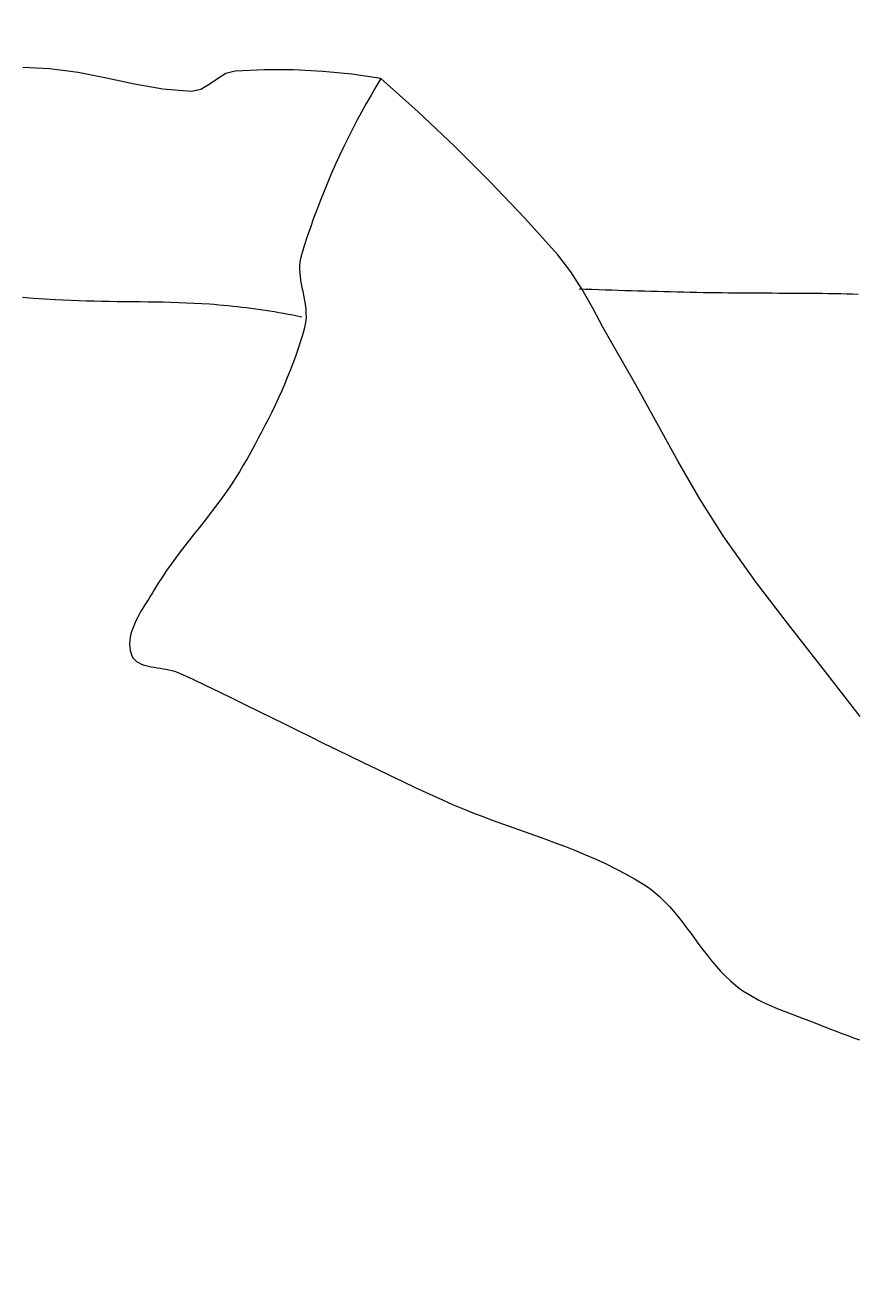
# Model space of a CAD drawing. Units: inches. Extents: x 1441 to 2460, y 1648 to 2683.
# Tile 6 of 35: x 1830 to 1852, y 1901 to 1933. Entities that reach past the tile are written whole.
import ezdxf

# ---------------------------------------------------------------- set-up
doc = ezdxf.new("R2010")
doc.units = ezdxf.units.IN
doc.layers.add('A-ANNO-DIMS', color=2, linetype='Continuous', lineweight=18)
doc.layers.add('A-FURN', color=8, linetype='Continuous', lineweight=15)
doc.styles.get("Standard").update_dxf_attribs({"font": 'arial.ttf'})
doc.dimstyles.get("Standard").update_dxf_attribs({"dimtxt": 0.18, "dimasz": 0.18, "dimexe": 0.18, "dimexo": 0.0625, "dimgap": 0.09, "dimtad": 0, "dimtih": 1, "dimtoh": 1, "dimdec": 4, "dimzin": 0, "dimdsep": 46, "dimtxsty": 'Standard', "dimcen": 0.09, "dimadec": 0, "dimazin": 0, "dimtfac": 1, "dimtdec": 4, "dimtofl": 0, "dimtmove": 0, "dimatfit": 3, "dimfxl": 1, "dimtolj": 1, "dimtzin": 0, "dimarcsym": 0})

# ---------------------------------------------------------------- blocks, each defined once
blk = doc.blocks.new('BED-DOUBLE-PLAN')
for p, q in [((5.86, 64.122), (5.863, 64.273)), ((16.787, 64.32), (15.632, 63.429)), ((25.038, 64.003), (25.093, 64.152)), ((25.093, 64.152), (25.148, 64.303)), ((5.849, 63.668), (5.852, 63.82)), ((5.852, 63.82), (5.856, 63.971)), ((5.856, 63.971), (5.86, 64.122)), ((24.925, 63.704), (24.982, 63.853)), ((24.982, 63.853), (25.038, 64.003)), ((5.843, 63.345), (5.846, 63.507)), ((5.846, 63.507), (5.849, 63.668)), ((24.81, 63.406), (24.868, 63.555)), ((24.868, 63.555), (24.925, 63.704)), ((5.839, 63.021), (5.841, 63.183)), ((5.841, 63.183), (5.843, 63.345)), ((15.632, 63.429), (14.485, 62.528)), ((24.707, 63.147), (24.751, 63.258)), ((24.751, 63.258), (24.81, 63.406)), ((5.837, 62.698), (5.838, 62.86)), ((5.838, 62.86), (5.839, 63.021)), ((24.579, 62.81), (24.621, 62.923)), ((24.621, 62.923), (24.664, 63.035)), ((24.664, 63.035), (24.707, 63.147)), ((5.835, 62.374), (5.836, 62.536)), ((5.836, 62.536), (5.837, 62.698)), ((14.485, 62.528), (13.327, 61.643)), ((24.452, 62.471), (24.495, 62.584)), ((24.495, 62.584), (24.537, 62.697)), ((24.537, 62.697), (24.579, 62.81)), ((5.834, 62.051), (5.835, 62.213)), ((5.835, 62.213), (5.835, 62.374)), ((24.319, 62.135), (24.364, 62.247)), ((24.364, 62.247), (24.409, 62.359)), ((24.409, 62.359), (24.452, 62.471)), ((5.833, 61.727), (5.834, 61.889)), ((5.834, 61.889), (5.834, 62.051)), ((24.172, 61.808), (24.223, 61.916)), ((24.223, 61.916), (24.271, 62.025)), ((24.271, 62.025), (24.319, 62.135)), ((5.832, 61.404), (5.833, 61.565)), ((5.833, 61.565), (5.833, 61.727)), ((13.327, 61.643), (12.139, 60.8)), ((24.004, 61.492), (24.063, 61.596)), ((24.063, 61.596), (24.119, 61.701)), ((24.119, 61.701), (24.172, 61.808)), ((5.83, 61.08), (5.831, 61.242)), ((5.831, 61.242), (5.832, 61.404)), ((23.737, 61.1), (23.809, 61.195)), ((23.809, 61.195), (23.878, 61.292)), ((23.878, 61.292), (23.943, 61.391)), ((23.943, 61.391), (24.004, 61.492)), ((5.826, 60.757), (5.828, 60.918)), ((5.828, 60.918), (5.83, 61.08)), ((23.502, 60.838), (23.623, 60.966)), ((23.623, 60.966), (23.737, 61.1)), ((5.821, 60.433), (5.824, 60.595)), ((5.824, 60.595), (5.826, 60.757)), ((12.139, 60.8), (11.176, 60.189)), ((23.108, 60.482), (23.244, 60.596)), ((23.244, 60.596), (23.376, 60.715)), ((23.376, 60.715), (23.502, 60.838)), ((5.815, 60.095), (5.818, 60.264)), ((5.818, 60.264), (5.821, 60.433)), ((22.683, 60.154), (22.826, 60.262)), ((22.826, 60.262), (22.968, 60.371)), ((22.968, 60.371), (23.108, 60.482)), ((5.807, 59.757), (5.811, 59.926)), ((5.811, 59.926), (5.815, 60.095)), ((11.176, 60.189), (10.189, 59.615)), ((22.249, 59.835), (22.393, 59.942)), ((22.393, 59.942), (22.538, 60.048)), ((22.538, 60.048), (22.683, 60.154)), ((5.799, 59.419), (5.803, 59.588)), ((5.803, 59.588), (5.807, 59.757)), ((10.189, 59.615), (9.189, 59.061)), ((21.83, 59.504), (21.967, 59.617)), ((21.967, 59.617), (22.107, 59.727)), ((22.107, 59.727), (22.249, 59.835)), ((5.791, 59.081), (5.795, 59.25)), ((5.795, 59.25), (5.799, 59.419)), ((21.449, 59.141), (21.571, 59.267)), ((21.571, 59.267), (21.698, 59.388)), ((21.698, 59.388), (21.83, 59.504)), ((5.782, 58.743), (5.786, 58.912)), ((5.786, 58.912), (5.791, 59.081)), ((9.189, 59.061), (8.189, 58.51)), ((21.227, 58.872), (21.335, 59.01)), ((21.335, 59.01), (21.449, 59.141)), ((5.772, 58.406), (5.777, 58.575)), ((5.777, 58.575), (5.782, 58.743)), ((20.982, 58.486), (21.129, 58.727)), ((21.129, 58.727), (21.227, 58.872)), ((5.767, 58.237), (5.772, 58.406)), ((8.189, 58.51), (7.197, 57.943)), ((20.844, 58.24), (20.982, 58.486)), ((5.756, 57.899), (5.761, 58.068)), ((5.761, 58.068), (5.767, 58.237)), ((7.197, 57.943), (6.716, 57.672)), ((20.59, 57.739), (20.714, 57.991)), ((20.714, 57.991), (20.844, 58.24)), ((5.744, 57.561), (5.75, 57.73)), ((5.75, 57.73), (5.756, 57.899)), ((6.716, 57.672), (6.229, 57.407)), ((20.473, 57.483), (20.59, 57.739)), ((5.732, 57.223), (5.738, 57.392)), ((5.738, 57.392), (5.744, 57.561)), ((6.229, 57.407), (5.748, 57.134)), ((20.361, 57.224), (20.473, 57.483)), ((5.748, 57.134), (5.285, 56.837)), ((5.726, 57.054), (5.732, 57.223)), ((20.15, 56.7), (20.254, 56.963)), ((20.254, 56.963), (20.361, 57.224)), ((5.285, 56.837), (4.851, 56.5)), ((20.05, 56.435), (20.15, 56.7)), ((4.851, 56.5), (3.888, 55.638)), ((19.952, 56.169), (20.05, 56.435)), ((19.856, 55.902), (19.952, 56.169)), ((3.888, 55.638), (2.949, 54.748)), ((19.666, 55.367), (19.761, 55.634)), ((19.761, 55.634), (19.856, 55.902)), ((19.571, 55.099), (19.666, 55.367)), ((19.474, 54.832), (19.571, 55.099)), ((2.949, 54.748), (2.036, 53.833)), ((19.375, 54.566), (19.474, 54.832)), ((19.274, 54.302), (19.375, 54.566)), ((19.059, 53.778), (19.169, 54.039)), ((19.169, 54.039), (19.274, 54.302)), ((2.036, 53.833), (1.148, 52.892)), ((18.945, 53.52), (19.059, 53.778)), ((18.788, 53.177), (18.945, 53.52)), ((18.629, 52.834), (18.788, 53.177)), ((1.148, 52.892), (0.288, 51.928)), ((18.468, 52.493), (18.629, 52.834)), ((18.306, 52.152), (18.468, 52.493)), ((18.143, 51.812), (18.306, 52.152)), ((0.288, 51.928), (0.178, 51.18)), ((0.288, 51.928), (0.502, 51.799)), ((0.502, 51.799), (0.719, 51.672)), ((17.979, 51.472), (18.143, 51.812)), ((0.719, 51.672), (0.936, 51.548)), ((0.936, 51.548), (1.156, 51.426)), ((1.156, 51.426), (1.377, 51.308)), ((17.814, 51.132), (17.979, 51.472)), ((0.178, 51.18), (0.104, 50.426)), ((1.377, 51.308), (1.6, 51.192)), ((1.6, 51.192), (1.824, 51.079)), ((1.824, 51.079), (2.05, 50.968)), ((17.648, 50.793), (17.814, 51.132)), ((2.05, 50.968), (2.277, 50.861)), ((2.277, 50.861), (2.505, 50.756)), ((2.505, 50.756), (2.735, 50.654)), ((17.481, 50.455), (17.648, 50.793)), ((0.104, 50.426), (0.065, 49.669)), ((2.735, 50.654), (2.966, 50.555)), ((2.966, 50.555), (3.198, 50.459)), ((3.198, 50.459), (3.432, 50.366)), ((17.314, 50.116), (17.481, 50.455)), ((3.432, 50.366), (3.666, 50.276)), ((3.666, 50.276), (3.901, 50.189)), ((3.901, 50.189), (4.138, 50.105)), ((4.138, 50.105), (4.375, 50.024)), ((17.147, 49.777), (17.314, 50.116)), ((4.375, 50.024), (4.613, 49.946)), ((4.613, 49.946), (4.852, 49.871)), ((4.852, 49.871), (4.943, 49.848)), ((4.943, 49.848), (5.034, 49.833)), ((5.034, 49.833), (5.127, 49.826)), ((5.127, 49.826), (5.22, 49.825)), ((5.22, 49.825), (5.314, 49.829)), ((5.314, 49.829), (5.409, 49.839)), ((5.409, 49.839), (5.504, 49.852)), ((5.504, 49.852), (5.6, 49.868)), ((5.6, 49.868), (5.695, 49.886)), ((5.695, 49.886), (5.791, 49.905)), ((5.791, 49.905), (5.887, 49.924)), ((5.887, 49.924), (5.983, 49.943)), ((5.983, 49.943), (6.079, 49.96)), ((6.079, 49.96), (6.174, 49.974)), ((6.174, 49.974), (6.269, 49.984)), ((6.269, 49.984), (6.363, 49.99)), ((6.363, 49.99), (6.457, 49.991)), ((6.436, 49.765), (6.412, 49.647)), ((6.46, 49.883), (6.436, 49.765)), ((6.457, 49.991), (6.55, 49.986)), ((6.55, 49.986), (6.643, 49.973)), ((6.643, 49.973), (6.734, 49.952)), ((6.734, 49.952), (6.921, 49.899)), ((6.921, 49.899), (7.107, 49.841)), ((7.107, 49.841), (7.292, 49.781)), ((7.292, 49.781), (7.476, 49.717)), ((16.98, 49.439), (17.147, 49.777)), ((0.065, 49.669), (0.062, 48.911)), ((6.39, 49.528), (6.368, 49.41)), ((6.412, 49.647), (6.39, 49.528)), ((7.476, 49.717), (7.659, 49.65)), ((7.659, 49.65), (7.841, 49.58)), ((7.841, 49.58), (8.022, 49.507)), ((8.022, 49.507), (8.202, 49.431)), ((8.202, 49.431), (8.381, 49.353)), ((16.813, 49.1), (16.98, 49.439)), ((6.326, 49.172), (6.307, 49.053)), ((6.347, 49.291), (6.326, 49.172)), ((6.368, 49.41), (6.347, 49.291)), ((8.381, 49.353), (8.56, 49.273)), ((8.56, 49.273), (8.737, 49.19)), ((8.737, 49.19), (8.913, 49.105)), ((8.913, 49.105), (9.088, 49.019)), ((16.647, 48.762), (16.813, 49.1)), ((0.062, 48.911), (0.095, 48.156)), ((6.27, 48.814), (6.253, 48.694)), ((6.288, 48.933), (6.27, 48.814)), ((6.307, 49.053), (6.288, 48.933)), ((9.088, 49.019), (9.263, 48.93)), ((9.263, 48.93), (9.436, 48.84)), ((9.436, 48.84), (9.609, 48.748)), ((16.481, 48.423), (16.647, 48.762)), ((6.221, 48.455), (6.207, 48.335)), ((6.237, 48.575), (6.221, 48.455)), ((6.253, 48.694), (6.237, 48.575)), ((9.609, 48.748), (9.781, 48.655)), ((9.781, 48.655), (9.952, 48.56)), ((9.952, 48.56), (10.122, 48.465)), ((10.122, 48.465), (10.291, 48.368)), ((0.095, 48.156), (0.161, 47.92)), ((6.193, 48.215), (6.18, 48.095)), ((6.207, 48.335), (6.193, 48.215)), ((10.291, 48.368), (10.462, 48.268)), ((10.462, 48.268), (10.629, 48.163)), ((10.629, 48.163), (10.794, 48.054)), ((16.315, 48.084), (16.481, 48.423)), ((0.161, 47.92), (0.294, 47.701)), ((6.156, 47.855), (6.146, 47.734)), ((6.168, 47.975), (6.156, 47.855)), ((6.18, 48.095), (6.168, 47.975)), ((10.794, 48.054), (10.957, 47.942)), ((10.957, 47.942), (11.118, 47.827)), ((11.118, 47.827), (11.277, 47.709)), ((16.151, 47.744), (16.315, 48.084)), ((0.294, 47.701), (0.446, 47.487)), ((0.446, 47.487), (0.571, 47.267)), ((6.127, 47.494), (6.114, 47.295)), ((6.136, 47.614), (6.127, 47.494)), ((6.146, 47.734), (6.136, 47.614)), ((11.277, 47.709), (11.435, 47.59)), ((11.435, 47.59), (11.593, 47.469)), ((11.593, 47.469), (11.749, 47.347)), ((15.987, 47.404), (16.151, 47.744)), ((0.571, 47.267), (0.62, 47.031)), ((6.114, 47.295), (6.104, 47.096)), ((11.749, 47.347), (11.905, 47.224)), ((11.905, 47.224), (12.061, 47.101)), ((15.824, 47.063), (15.987, 47.404)), ((0.62, 47.031), (0.562, 46.291)), ((6.095, 46.897), (6.087, 46.698)), ((6.104, 47.096), (6.095, 46.897)), ((12.061, 47.101), (12.218, 46.979)), ((12.218, 46.979), (12.374, 46.857)), ((12.374, 46.857), (12.532, 46.737)), ((15.663, 46.722), (15.824, 47.063)), ((6.081, 46.499), (6.076, 46.3)), ((6.087, 46.698), (6.081, 46.499)), ((12.532, 46.737), (12.691, 46.618)), ((12.691, 46.618), (12.851, 46.501)), ((12.851, 46.501), (13.012, 46.387)), ((15.578, 46.447), (15.595, 46.52)), ((15.595, 46.52), (15.614, 46.591)), ((15.614, 46.591), (15.636, 46.659)), ((15.636, 46.659), (15.663, 46.722)), ((0.562, 46.291), (0.434, 45.558)), ((6.076, 46.3), (6.072, 46.1)), ((13.012, 46.387), (13.176, 46.276)), ((13.176, 46.276), (13.342, 46.169)), ((13.342, 46.169), (13.511, 46.065)), ((15.515, 46.065), (15.527, 46.141)), ((15.527, 46.141), (15.539, 46.218)), ((15.539, 46.218), (15.551, 46.295)), ((15.551, 46.295), (15.564, 46.372)), ((15.564, 46.372), (15.578, 46.447)), ((6.069, 45.901), (6.067, 45.702)), ((6.072, 46.1), (6.069, 45.901)), ((13.511, 46.065), (13.587, 46.019)), ((13.587, 46.019), (13.664, 45.971)), ((13.664, 45.971), (13.742, 45.922)), ((13.742, 45.922), (13.822, 45.871)), ((13.822, 45.871), (13.902, 45.821)), ((13.902, 45.821), (13.983, 45.771)), ((15.448, 45.78), (15.468, 45.847)), ((15.468, 45.847), (15.486, 45.917)), ((15.486, 45.917), (15.502, 45.99)), ((15.502, 45.99), (15.515, 46.065)), ((0.434, 45.558), (0.277, 44.827)), ((6.064, 45.502), (6.062, 45.303)), ((6.067, 45.702), (6.064, 45.502)), ((13.983, 45.771), (14.065, 45.723)), ((14.065, 45.723), (14.147, 45.676)), ((14.147, 45.676), (14.231, 45.631)), ((14.231, 45.631), (14.314, 45.589)), ((14.314, 45.589), (14.398, 45.551)), ((14.398, 45.551), (14.483, 45.517)), ((14.483, 45.517), (14.567, 45.487)), ((14.567, 45.487), (14.652, 45.463)), ((15.16, 45.466), (15.221, 45.49)), ((15.221, 45.49), (15.274, 45.522)), ((15.274, 45.522), (15.32, 45.561)), ((15.32, 45.561), (15.36, 45.608)), ((15.36, 45.608), (15.394, 45.66)), ((15.394, 45.66), (15.423, 45.718)), ((15.423, 45.718), (15.448, 45.78)), ((6.062, 45.303), (6.06, 45.104)), ((14.652, 45.463), (14.737, 45.445)), ((14.737, 45.445), (14.822, 45.434)), ((14.822, 45.434), (14.907, 45.429)), ((14.907, 45.429), (14.992, 45.433)), ((14.992, 45.433), (15.076, 45.445)), ((15.076, 45.445), (15.16, 45.466)), ((6.057, 44.904), (6.054, 44.705)), ((6.06, 45.104), (6.057, 44.904)), ((0.277, 44.827), (0.13, 44.094)), ((6.05, 44.506), (6.045, 44.306)), ((6.054, 44.705), (6.05, 44.506)), ((6.045, 44.306), (6.039, 44.107)), ((0.13, 44.094), (0.035, 43.356)), ((6.031, 43.908), (6.022, 43.709)), ((6.039, 44.107), (6.031, 43.908)), ((6.022, 43.709), (6.011, 43.51)), ((0.035, 43.356), (0.002, 42.668)), ((5.993, 43.227), (5.975, 42.943)), ((6.011, 43.51), (5.993, 43.227)), ((5.975, 42.943), (5.955, 42.66))]:
    blk.add_line(p, q)
blk = doc.blocks.new('*D67')
at = {"layer": 'A-ANNO-DIMS', "color": 0, "lineweight": -2, "transparency": 16777216}
for p, q in [((1889.448, 2298.695), (1916.216, 2298.695)), ((1916.036, 2298.515), (1916.036, 2055.938)), ((1916.036, 1812.997), (1916.036, 2055.574)), ((1758.224, 1812.817), (1916.216, 1812.817))]:
    blk.add_line(p, q, dxfattribs=at)
at = {"layer": 'A-ANNO-DIMS', "color": 0, "transparency": 16777216}
for points in [[(1916.006, 2298.515), (1916.066, 2298.515), (1916.036, 2298.695)], [(1916.006, 1812.997), (1916.066, 1812.997), (1916.036, 1812.817)]]:
    blk.add_solid(points, dxfattribs=at)
at = {"layer": 'Defpoints', "color": 0, "transparency": 16777216}
for p in [(1889.386, 2298.695), (1916.036, 2298.695), (1758.161, 1812.817)]:
    blk.add_point(p, dxfattribs=at)
at = {"layer": 'A-ANNO-DIMS', "color": 0, "transparency": 16777216, "insert": (1916.036, 2055.756), "char_height": 0.18, "attachment_point": 5}
blk.add_mtext('\\A1;485.9', dxfattribs=at)

msp = doc.modelspace()

# ---------------------------------------------------------------- block references
at = {"layer": 'A-FURN', "rotation": 270}
msp.add_blockref('BED-DOUBLE-PLAN', (1787.6309, 1932.2861), dxfattribs=at)

# ---------------------------------------------------------------- dimensions: what is measured, and where the dimension line sits
at = {"layer": 'A-ANNO-DIMS'}
dim = msp.add_linear_dim(base=(1916.0359, 2298.6952), p1=(1758.1615, 1812.8171), p2=(1889.3859, 2298.6952), angle=90, dimstyle='Standard', override={"dimdec": 1, "dimlfac": 1, "dimrnd": 0, "dimzin": 0, "dimdsep": 46, "dimlunit": 2}, dxfattribs=at)
dim.commit()
dim.dimension.update_dxf_attribs({"geometry": '*D67', "text_midpoint": (1916.0359, 2055.7561)})

doc.saveas('drawing.dxf')
